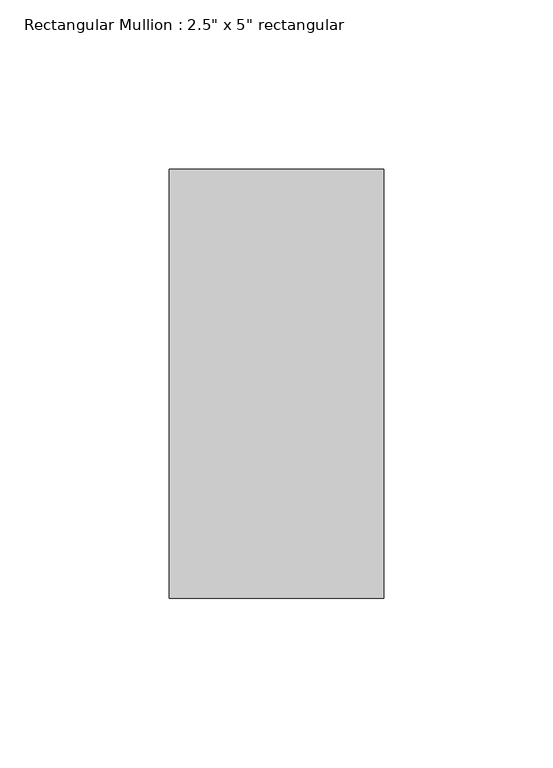
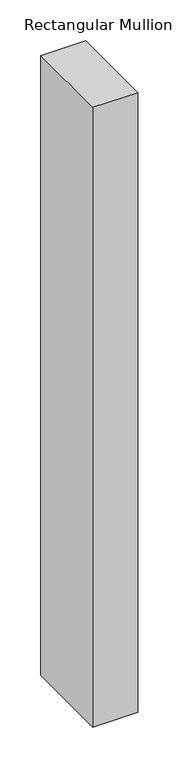
"""IFC4 building model written with IfcOpenShell, lengths in millimetres: member geometry."""

from ifc_helpers import new_model, si_unit, frame, origin, place, context, project, spatial, polyline, outline, extrude, source, transform, mapped, element, save


def member_b0b512a9(model_context):
    return source(origin(), model_context, "Body", "SweptSolid", [
        extrude(outline(polyline([(0.0, 63.5), (0.0, -63.5), (-63.5, -63.5), (-63.5, 63.5), (0.0, 63.5)])), frame((0.0, 0.0, -924.7594531), z_axis=(0.0, 0.0, 1.0), x_axis=(1.0, 0.0, 0.0)), (0.0, 0.0, 1.0), 924.7594531),
    ])


if __name__ == "__main__":
    model = new_model("IFC4")
    model_context = context("Model", 3, world=origin())
    ifc_project = project(units=[si_unit("LENGTHUNIT", "METRE", prefix="MILLI")], contexts=[model_context])
    site = spatial("IfcSite", under=ifc_project)
    building = spatial("IfcBuilding", under=site)
    placement = place(None, origin())
    member_shape = member_b0b512a9(model_context)
    element("IfcMember", 1, ObjectType="Rectangular Mullion : 2.5\" x 5\" rectangular", at=placement, inside=building, context=model_context, shape_type="MappedRepresentation", body=[
        mapped(member_shape, transform((0.0, 0.0, 0.0), x_axis=(1.0, 0.0, 0.0), y_axis=(0.0, 1.0, 0.0), z_axis=(0.0, 0.0, 1.0))),
    ])
    save(model, "model.ifc")

# Revit data of these elements
# Type "Rectangular Mullion : 2.5\" x 5\" rectangular"
#   built-in parameter 1007304 = 0.416667 (stored number, unit not read)
#   built-in parameter 1007301 = 0.104167 (stored number, unit not read)
#   built-in parameter 1007300 = 0.104167 (stored number, unit not read)
# Element 1 (IfcMember, "Rectangular Mullion : 2.5\" x 5\" rectangular")
#   Materials on its faces: "Aluminum"
# Materials
#   "Aluminum": class "Metal", colour RGB 247 247 247, transparency 0, Description = "Aluminum 6061", Cost = 0
